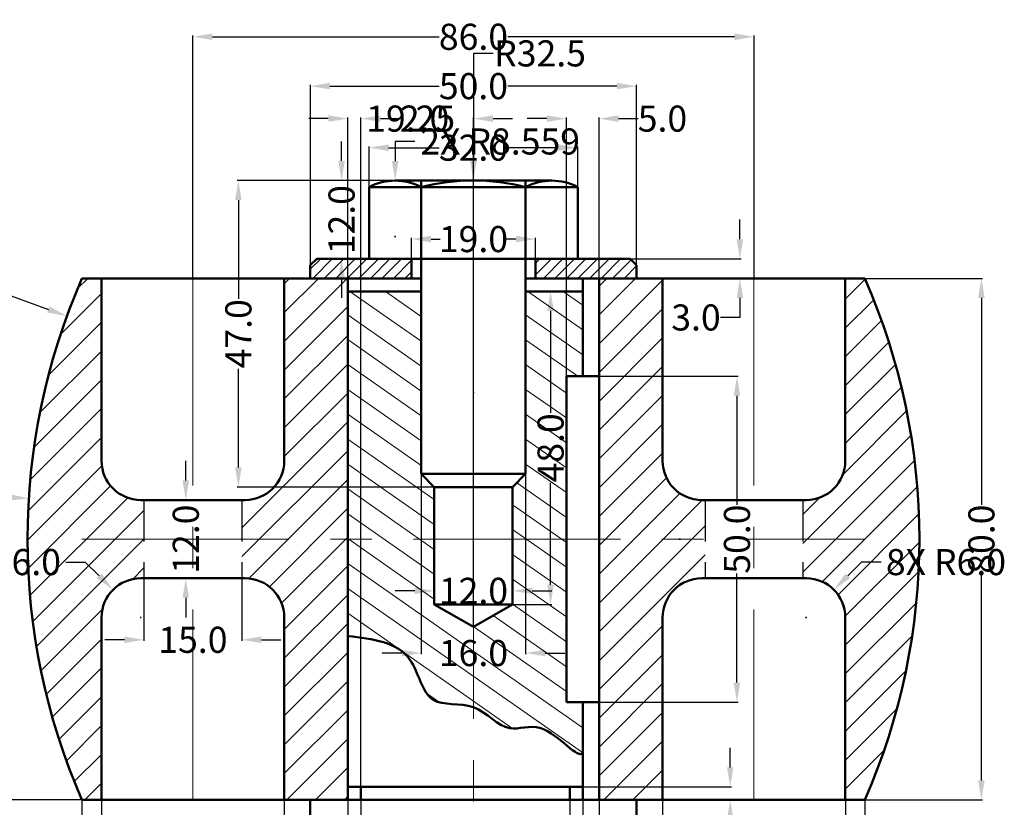
# Model space of a CAD drawing. Units: millimetres. Extents: x 285 to 514, y 588 to 771.
# Tile 3 of 3: x 363 to 514, y 650 to 771. Entities that reach past the tile are written whole.
import ezdxf

# ---------------------------------------------------------------- set-up
doc = ezdxf.new("R2010")
doc.units = ezdxf.units.MM
doc.header["$MEASUREMENT"] = 0
doc.linetypes.add('CENTER', pattern=[50.8, 31.75, -6.35, 6.35, -6.35])
doc.linetypes.add('HIDDEN', pattern=[9.525, 6.35, -3.175])
for name, color, linetype, lineweight in [('M-CNTR', 1, 'CENTER', 18), ('M-DIMS', 2, 'Continuous', 25), ('M-HATC', 8, 'Continuous', 18), ('M-HIDN', 3, 'HIDDEN', 25), ('M-OUTL', 7, 'Continuous', 50)]:
    doc.layers.add(name, color=color, linetype=linetype, lineweight=lineweight)
doc.styles.get("Standard").update_dxf_attribs({"font": 'arial.ttf'})
doc.dimstyles.get("Standard").update_dxf_attribs({"dimtxt": 4, "dimasz": 3, "dimexe": 0.18, "dimexo": 0.0625, "dimgap": 0.09, "dimtad": 0, "dimtoh": 1, "dimdec": 1, "dimzin": 0, "dimdsep": 46, "dimtxsty": 'Standard', "dimcen": 0.09, "dimadec": 0, "dimazin": 0, "dimtfac": 1, "dimtdec": 1, "dimtofl": 0, "dimtmove": 0, "dimatfit": 3, "dimfxl": 1, "dimtolj": 1, "dimtzin": 0, "dimarcsym": 0})

# ---------------------------------------------------------------- blocks, each defined once
blk = doc.blocks.new('*D1')
at = {"layer": 'Defpoints', "color": 0, "transparency": 16777216}
for p in [(413.04, 651.15), (451.54, 651.15), (451.54, 632.52)]:
    blk.add_point(p, dxfattribs=at)
at = {"layer": 'M-DIMS', "color": 0, "lineweight": -2, "transparency": 16777216}
for p, q in [((413.04, 651.09), (413.04, 632.34)), ((451.54, 651.09), (451.54, 632.34)), ((416.04, 632.52), (426.99, 632.52)), ((448.54, 632.52), (437.59, 632.52))]:
    blk.add_line(p, q, dxfattribs=at)
at = {"layer": 'M-DIMS', "color": 0, "transparency": 16777216}
for points in [[(416.04, 633.02), (416.04, 632.02), (413.04, 632.52)], [(448.54, 633.02), (448.54, 632.02), (451.54, 632.52)]]:
    blk.add_solid(points, dxfattribs=at)
at = {"layer": 'M-DIMS', "color": 0, "transparency": 16777216, "insert": (432.29, 632.52), "char_height": 4, "attachment_point": 5}
blk.add_mtext('\\A1;38.5', dxfattribs=at)
blk = doc.blocks.new('*D2')
at = {"layer": 'Defpoints', "color": 0, "transparency": 16777216}
for p in [(449.04, 656.31), (413.04, 648.81), (449.04, 638.14)]:
    blk.add_point(p, dxfattribs=at)
at = {"layer": 'M-DIMS', "color": 0, "lineweight": -2, "transparency": 16777216}
for p, q in [((449.04, 656.25), (449.04, 637.96)), ((413.04, 648.75), (413.04, 637.96)), ((416.04, 638.14), (425.76, 638.14)), ((446.04, 638.14), (436.31, 638.14))]:
    blk.add_line(p, q, dxfattribs=at)
at = {"layer": 'M-DIMS', "color": 0, "transparency": 16777216}
for points in [[(416.04, 638.64), (416.04, 637.64), (413.04, 638.14)], [(446.04, 638.64), (446.04, 637.64), (449.04, 638.14)]]:
    blk.add_solid(points, dxfattribs=at)
at = {"layer": 'M-DIMS', "color": 0, "transparency": 16777216, "insert": (431.04, 638.14), "char_height": 4, "attachment_point": 5}
blk.add_mtext('\\A1;36.0', dxfattribs=at)
blk = doc.blocks.new('*D3')
at = {"layer": 'Defpoints', "color": 0, "transparency": 16777216}
for p in [(364.13, 697.39), (463.94, 691.15)]:
    blk.add_point(p, dxfattribs=at)
at = {"layer": 'M-DIMS', "color": 0, "lineweight": -2, "transparency": 16777216}
for p, q in [((337.25, 699.07), (361.14, 697.58)), ((463.94, 691.06), (463.94, 691.24)), ((463.85, 691.15), (464.03, 691.15))]:
    blk.add_line(p, q, dxfattribs=at)
at = {"layer": 'M-DIMS', "color": 0, "transparency": 16777216}
blk.add_solid([(361.17, 698.07), (361.11, 697.08), (364.13, 697.39)], dxfattribs=at)
at = {"layer": 'M-DIMS', "color": 0, "transparency": 16777216, "insert": (328.5, 699.07), "char_height": 4, "attachment_point": 5}
blk.add_mtext('\\A1;R100.0', dxfattribs=at)
blk = doc.blocks.new('*D4')
at = {"layer": 'Defpoints', "color": 0, "transparency": 16777216}
for p in [(372.29, 651.15), (492.29, 651.15), (492.29, 590.54)]:
    blk.add_point(p, dxfattribs=at)
at = {"layer": 'M-DIMS', "color": 0, "lineweight": -2, "transparency": 16777216}
for p, q in [((372.29, 651.09), (372.29, 590.36)), ((492.29, 651.09), (492.29, 590.36)), ((375.29, 590.54), (425.64, 590.54)), ((489.29, 590.54), (438.93, 590.54))]:
    blk.add_line(p, q, dxfattribs=at)
at = {"layer": 'M-DIMS', "color": 0, "transparency": 16777216}
for points in [[(375.29, 591.04), (375.29, 590.04), (372.29, 590.54)], [(489.29, 591.04), (489.29, 590.04), (492.29, 590.54)]]:
    blk.add_solid(points, dxfattribs=at)
at = {"layer": 'M-DIMS', "color": 0, "transparency": 16777216, "insert": (432.29, 590.54), "char_height": 4, "attachment_point": 5}
blk.add_mtext('\\A1;120.0', dxfattribs=at)
blk = doc.blocks.new('*D5')
at = {"layer": 'Defpoints', "color": 0, "transparency": 16777216}
for p in [(375.29, 651.15), (489.29, 651.15), (489.29, 598.24)]:
    blk.add_point(p, dxfattribs=at)
at = {"layer": 'M-DIMS', "color": 0, "lineweight": -2, "transparency": 16777216}
for p, q in [((375.29, 651.09), (375.29, 598.06)), ((489.29, 651.09), (489.29, 598.06)), ((378.29, 598.24), (425.64, 598.24)), ((486.29, 598.24), (438.93, 598.24))]:
    blk.add_line(p, q, dxfattribs=at)
at = {"layer": 'M-DIMS', "color": 0, "transparency": 16777216}
for points in [[(378.29, 598.74), (378.29, 597.74), (375.29, 598.24)], [(486.29, 598.74), (486.29, 597.74), (489.29, 598.24)]]:
    blk.add_solid(points, dxfattribs=at)
at = {"layer": 'M-DIMS', "color": 0, "transparency": 16777216, "insert": (432.29, 598.24), "char_height": 4, "attachment_point": 5}
blk.add_mtext('\\A1;114.0', dxfattribs=at)
blk = doc.blocks.new('*D6')
at = {"layer": 'Defpoints', "color": 0, "transparency": 16777216}
for p in [(403.29, 651.15), (461.29, 651.15), (461.29, 604.76)]:
    blk.add_point(p, dxfattribs=at)
at = {"layer": 'M-DIMS', "color": 0, "lineweight": -2, "transparency": 16777216}
for p, q in [((403.29, 651.09), (403.29, 604.58)), ((461.29, 651.09), (461.29, 604.58)), ((406.29, 604.76), (427.01, 604.76)), ((458.29, 604.76), (437.57, 604.76))]:
    blk.add_line(p, q, dxfattribs=at)
at = {"layer": 'M-DIMS', "color": 0, "transparency": 16777216}
for points in [[(406.29, 605.26), (406.29, 604.26), (403.29, 604.76)], [(458.29, 605.26), (458.29, 604.26), (461.29, 604.76)]]:
    blk.add_solid(points, dxfattribs=at)
at = {"layer": 'M-DIMS', "color": 0, "transparency": 16777216, "insert": (432.29, 604.76), "char_height": 4, "attachment_point": 5}
blk.add_mtext('\\A1;58.0', dxfattribs=at)
blk = doc.blocks.new('*D8')
at = {"layer": 'Defpoints', "color": 0, "transparency": 16777216}
for p in [(415.04, 651.15), (447.04, 651.15), (447.04, 644.96)]:
    blk.add_point(p, dxfattribs=at)
at = {"layer": 'M-DIMS', "color": 0, "lineweight": -2, "transparency": 16777216}
for p, q in [((415.04, 651.09), (415.04, 644.78)), ((447.04, 651.09), (447.04, 644.78)), ((418.04, 644.96), (425.76, 644.96)), ((444.04, 644.96), (436.31, 644.96))]:
    blk.add_line(p, q, dxfattribs=at)
at = {"layer": 'M-DIMS', "color": 0, "transparency": 16777216}
for points in [[(418.04, 645.46), (418.04, 644.46), (415.04, 644.96)], [(444.04, 645.46), (444.04, 644.46), (447.04, 644.96)]]:
    blk.add_solid(points, dxfattribs=at)
at = {"layer": 'M-DIMS', "color": 0, "transparency": 16777216, "insert": (431.04, 644.96), "char_height": 4, "attachment_point": 5}
blk.add_mtext('\\A1;32.0', dxfattribs=at)
blk = doc.blocks.new('*D9')
at = {"layer": 'Defpoints', "color": 0, "transparency": 16777216}
for p in [(381.79, 685.15), (396.79, 685.15), (396.79, 675.71)]:
    blk.add_point(p, dxfattribs=at)
at = {"layer": 'M-DIMS', "color": 0, "lineweight": -2, "transparency": 16777216}
for p, q in [((381.79, 685.09), (381.79, 675.53)), ((396.79, 685.09), (396.79, 675.53)), ((378.79, 675.71), (375.79, 675.71)), ((399.79, 675.71), (402.79, 675.71))]:
    blk.add_line(p, q, dxfattribs=at)
at = {"layer": 'M-DIMS', "color": 0, "transparency": 16777216}
for points in [[(378.79, 676.21), (378.79, 675.21), (381.79, 675.71)], [(399.79, 676.21), (399.79, 675.21), (396.79, 675.71)]]:
    blk.add_solid(points, dxfattribs=at)
at = {"layer": 'M-DIMS', "color": 0, "transparency": 16777216, "insert": (389.29, 675.71), "char_height": 4, "attachment_point": 5}
blk.add_mtext('\\A1;15.0', dxfattribs=at)
blk = doc.blocks.new('*D10')
at = {"layer": 'Defpoints', "color": 0, "transparency": 16777216}
for p in [(424.29, 746.15), (412.07, 734.15), (424.29, 734.15)]:
    blk.add_point(p, dxfattribs=at)
at = {"layer": 'M-DIMS', "color": 0, "lineweight": -2, "transparency": 16777216}
for p, q in [((412.07, 749.15), (412.07, 752.15)), ((424.22, 746.15), (411.89, 746.15)), ((424.22, 734.15), (411.89, 734.15)), ((412.07, 731.15), (412.07, 728.15))]:
    blk.add_line(p, q, dxfattribs=at)
at = {"layer": 'M-DIMS', "color": 0, "transparency": 16777216}
for points in [[(411.57, 749.15), (412.57, 749.15), (412.07, 746.15)], [(411.57, 731.15), (412.57, 731.15), (412.07, 734.15)]]:
    blk.add_solid(points, dxfattribs=at)
at = {"layer": 'M-DIMS', "color": 0, "transparency": 16777216, "insert": (412.07, 740.15), "char_height": 4, "attachment_point": 5, "rotation": 90}
blk.add_mtext('\\A1;12.0', dxfattribs=at)
blk = doc.blocks.new('*D11')
at = {"layer": 'Defpoints', "color": 0, "transparency": 16777216}
for p in [(416.29, 746.15), (396.26, 699.14), (426.29, 699.14)]:
    blk.add_point(p, dxfattribs=at)
at = {"layer": 'M-DIMS', "color": 0, "lineweight": -2, "transparency": 16777216}
for p, q in [((416.23, 746.15), (396.08, 746.15)), ((396.26, 743.15), (396.26, 728)), ((396.26, 702.14), (396.26, 717.29)), ((426.22, 699.14), (396.08, 699.14))]:
    blk.add_line(p, q, dxfattribs=at)
at = {"layer": 'M-DIMS', "color": 0, "transparency": 16777216}
for points in [[(395.76, 743.15), (396.76, 743.15), (396.26, 746.15)], [(395.76, 702.14), (396.76, 702.14), (396.26, 699.14)]]:
    blk.add_solid(points, dxfattribs=at)
at = {"layer": 'M-DIMS', "color": 0, "transparency": 16777216, "insert": (396.26, 722.65), "char_height": 4, "attachment_point": 5, "rotation": 90}
blk.add_mtext('\\A1;47.0', dxfattribs=at)
blk = doc.blocks.new('*D12')
at = {"layer": 'Defpoints', "color": 0, "transparency": 16777216}
for p in [(475.29, 768.2), (389.29, 731.15), (475.29, 731.15)]:
    blk.add_point(p, dxfattribs=at)
at = {"layer": 'M-DIMS', "color": 0, "lineweight": -2, "transparency": 16777216}
for p, q in [((389.29, 731.21), (389.29, 768.38)), ((392.29, 768.2), (427.01, 768.2)), ((472.29, 768.2), (437.57, 768.2)), ((475.29, 731.21), (475.29, 768.38))]:
    blk.add_line(p, q, dxfattribs=at)
at = {"layer": 'M-DIMS', "color": 0, "transparency": 16777216}
for points in [[(392.29, 768.7), (392.29, 767.7), (389.29, 768.2)], [(472.29, 768.7), (472.29, 767.7), (475.29, 768.2)]]:
    blk.add_solid(points, dxfattribs=at)
at = {"layer": 'M-DIMS', "color": 0, "transparency": 16777216, "insert": (432.29, 768.2), "char_height": 4, "attachment_point": 5}
blk.add_mtext('\\A1;86.0', dxfattribs=at)
blk = doc.blocks.new('*D13')
at = {"layer": 'Defpoints', "color": 0, "transparency": 16777216}
for p in [(448.29, 751.19), (416.29, 742.48), (448.29, 742.48)]:
    blk.add_point(p, dxfattribs=at)
at = {"layer": 'M-DIMS', "color": 0, "lineweight": -2, "transparency": 16777216}
for p, q in [((416.29, 742.54), (416.29, 751.37)), ((419.29, 751.19), (427.01, 751.19)), ((445.29, 751.19), (437.56, 751.19)), ((448.29, 742.54), (448.29, 751.37))]:
    blk.add_line(p, q, dxfattribs=at)
at = {"layer": 'M-DIMS', "color": 0, "transparency": 16777216}
for points in [[(419.29, 751.69), (419.29, 750.69), (416.29, 751.19)], [(445.29, 751.69), (445.29, 750.69), (448.29, 751.19)]]:
    blk.add_solid(points, dxfattribs=at)
at = {"layer": 'M-DIMS', "color": 0, "transparency": 16777216, "insert": (432.29, 751.19), "char_height": 4, "attachment_point": 5}
blk.add_mtext('\\A1;32.0', dxfattribs=at)
blk = doc.blocks.new('*D14')
at = {"layer": 'Defpoints', "color": 0, "transparency": 16777216}
for p in [(457.29, 760.63), (407.29, 731.15), (457.29, 731.15)]:
    blk.add_point(p, dxfattribs=at)
at = {"layer": 'M-DIMS', "color": 0, "lineweight": -2, "transparency": 16777216}
for p, q in [((407.29, 731.21), (407.29, 760.81)), ((410.29, 760.63), (427.01, 760.63)), ((454.29, 760.63), (437.57, 760.63)), ((457.29, 731.21), (457.29, 760.81))]:
    blk.add_line(p, q, dxfattribs=at)
at = {"layer": 'M-DIMS', "color": 0, "transparency": 16777216}
for points in [[(410.29, 761.13), (410.29, 760.13), (407.29, 760.63)], [(454.29, 761.13), (454.29, 760.13), (457.29, 760.63)]]:
    blk.add_solid(points, dxfattribs=at)
at = {"layer": 'M-DIMS', "color": 0, "transparency": 16777216, "insert": (432.29, 760.63), "char_height": 4, "attachment_point": 5}
blk.add_mtext('\\A1;50.0', dxfattribs=at)
blk = doc.blocks.new('*D15')
at = {"layer": 'Defpoints', "color": 0, "transparency": 16777216}
for p in [(444.66, 729.15), (438.29, 681.15), (444.11, 681.15)]:
    blk.add_point(p, dxfattribs=at)
at = {"layer": 'M-DIMS', "color": 0, "lineweight": -2, "transparency": 16777216}
for p, q in [((444.6, 729.15), (443.93, 729.15)), ((444.11, 726.15), (444.11, 710.51)), ((444.11, 684.15), (444.11, 699.79)), ((438.35, 681.15), (444.29, 681.15))]:
    blk.add_line(p, q, dxfattribs=at)
at = {"layer": 'M-DIMS', "color": 0, "transparency": 16777216}
for points in [[(443.61, 726.15), (444.61, 726.15), (444.11, 729.15)], [(443.61, 684.15), (444.61, 684.15), (444.11, 681.15)]]:
    blk.add_solid(points, dxfattribs=at)
at = {"layer": 'M-DIMS', "color": 0, "transparency": 16777216, "insert": (444.11, 705.15), "char_height": 4, "attachment_point": 5, "rotation": 90}
blk.add_mtext('\\A1;48.0', dxfattribs=at)
blk = doc.blocks.new('*D16')
at = {"layer": 'Defpoints', "color": 0, "transparency": 16777216}
for p in [(424.29, 701.14), (440.29, 701.14), (440.29, 673.68)]:
    blk.add_point(p, dxfattribs=at)
at = {"layer": 'M-DIMS', "color": 0, "lineweight": -2, "transparency": 16777216}
for p, q in [((424.29, 701.08), (424.29, 673.5)), ((440.29, 701.08), (440.29, 673.5)), ((421.29, 673.68), (418.29, 673.68)), ((443.29, 673.68), (446.29, 673.68))]:
    blk.add_line(p, q, dxfattribs=at)
at = {"layer": 'M-DIMS', "color": 0, "transparency": 16777216}
for points in [[(421.29, 674.18), (421.29, 673.18), (424.29, 673.68)], [(443.29, 674.18), (443.29, 673.18), (440.29, 673.68)]]:
    blk.add_solid(points, dxfattribs=at)
at = {"layer": 'M-DIMS', "color": 0, "transparency": 16777216, "insert": (432.29, 673.68), "char_height": 4, "attachment_point": 5}
blk.add_mtext('\\A1;16.0', dxfattribs=at)
blk = doc.blocks.new('*D17')
at = {"layer": 'Defpoints', "color": 0, "transparency": 16777216}
for p in [(438.29, 683.22), (426.29, 681.15), (438.29, 681.15)]:
    blk.add_point(p, dxfattribs=at)
at = {"layer": 'M-DIMS', "color": 0, "lineweight": -2, "transparency": 16777216}
for p, q in [((423.29, 683.22), (420.29, 683.22)), ((426.29, 681.21), (426.29, 683.4)), ((438.29, 681.21), (438.29, 683.4)), ((441.29, 683.22), (444.29, 683.22))]:
    blk.add_line(p, q, dxfattribs=at)
at = {"layer": 'M-DIMS', "color": 0, "transparency": 16777216}
for points in [[(423.29, 683.72), (423.29, 682.72), (426.29, 683.22)], [(441.29, 683.72), (441.29, 682.72), (438.29, 683.22)]]:
    blk.add_solid(points, dxfattribs=at)
at = {"layer": 'M-DIMS', "color": 0, "transparency": 16777216, "insert": (432.29, 683.22), "char_height": 4, "attachment_point": 5}
blk.add_mtext('\\A1;12.0', dxfattribs=at)
blk = doc.blocks.new('*D18')
at = {"layer": 'Defpoints', "color": 0, "transparency": 16777216}
for p in [(451.54, 716.15), (451.54, 666.15), (472.68, 666.15)]:
    blk.add_point(p, dxfattribs=at)
at = {"layer": 'M-DIMS', "color": 0, "lineweight": -2, "transparency": 16777216}
for p, q in [((451.6, 716.15), (472.86, 716.15)), ((472.68, 713.15), (472.68, 696.43)), ((472.68, 669.15), (472.68, 685.87)), ((451.6, 666.15), (472.86, 666.15))]:
    blk.add_line(p, q, dxfattribs=at)
at = {"layer": 'M-DIMS', "color": 0, "transparency": 16777216}
for points in [[(472.18, 713.15), (473.18, 713.15), (472.68, 716.15)], [(472.18, 669.15), (473.18, 669.15), (472.68, 666.15)]]:
    blk.add_solid(points, dxfattribs=at)
at = {"layer": 'M-DIMS', "color": 0, "transparency": 16777216, "insert": (472.68, 691.15), "char_height": 4, "attachment_point": 5, "rotation": 90}
blk.add_mtext('\\A1;50.0', dxfattribs=at)
blk = doc.blocks.new('*D19')
at = {"layer": 'Defpoints', "color": 0, "transparency": 16777216}
for p in [(449.04, 653.15), (449.04, 651.15), (471.64, 651.15)]:
    blk.add_point(p, dxfattribs=at)
at = {"layer": 'M-DIMS', "color": 0, "lineweight": -2, "transparency": 16777216}
for p, q in [((471.64, 656.15), (471.64, 659.15)), ((449.1, 653.15), (471.82, 653.15)), ((449.1, 651.15), (471.82, 651.15)), ((471.64, 648.15), (471.64, 645.15)), ((471.64, 645.15), (468.64, 645.15))]:
    blk.add_line(p, q, dxfattribs=at)
at = {"layer": 'M-DIMS', "color": 0, "transparency": 16777216}
for points in [[(471.14, 656.15), (472.14, 656.15), (471.64, 653.15)], [(471.14, 648.15), (472.14, 648.15), (471.64, 651.15)]]:
    blk.add_solid(points, dxfattribs=at)
at = {"layer": 'M-DIMS', "color": 0, "transparency": 16777216, "insert": (464.88, 645.15), "char_height": 4, "attachment_point": 5}
blk.add_mtext('\\A1;2.0', dxfattribs=at)
blk = doc.blocks.new('*D20')
at = {"layer": 'Defpoints', "color": 0, "transparency": 16777216}
for p in [(455.38, 734.15), (455.38, 731.15), (473.13, 731.15)]:
    blk.add_point(p, dxfattribs=at)
at = {"layer": 'M-DIMS', "color": 0, "lineweight": -2, "transparency": 16777216}
for p, q in [((473.13, 737.15), (473.13, 740.15)), ((455.44, 734.15), (473.31, 734.15)), ((455.44, 731.15), (473.31, 731.15)), ((473.13, 728.15), (473.13, 725.15)), ((473.13, 725.15), (470.13, 725.15))]:
    blk.add_line(p, q, dxfattribs=at)
at = {"layer": 'M-DIMS', "color": 0, "transparency": 16777216}
for points in [[(472.63, 737.15), (473.63, 737.15), (473.13, 734.15)], [(472.63, 728.15), (473.63, 728.15), (473.13, 731.15)]]:
    blk.add_solid(points, dxfattribs=at)
at = {"layer": 'M-DIMS', "color": 0, "transparency": 16777216, "insert": (466.4, 725.15), "char_height": 4, "attachment_point": 5}
blk.add_mtext('\\A1;3.0', dxfattribs=at)
blk = doc.blocks.new('*D21')
at = {"layer": 'Defpoints', "color": 0, "transparency": 16777216}
for p in [(441.79, 737.17), (422.79, 732.58), (441.79, 732.65)]:
    blk.add_point(p, dxfattribs=at)
at = {"layer": 'M-DIMS', "color": 0, "lineweight": -2, "transparency": 16777216}
for p, q in [((422.79, 732.64), (422.79, 737.35)), ((425.79, 737.17), (427.2, 737.17)), ((438.79, 737.17), (437.38, 737.17)), ((441.79, 732.71), (441.79, 737.35))]:
    blk.add_line(p, q, dxfattribs=at)
at = {"layer": 'M-DIMS', "color": 0, "transparency": 16777216}
for points in [[(425.79, 737.67), (425.79, 736.67), (422.79, 737.17)], [(438.79, 737.67), (438.79, 736.67), (441.79, 737.17)]]:
    blk.add_solid(points, dxfattribs=at)
at = {"layer": 'M-DIMS', "color": 0, "transparency": 16777216, "insert": (432.29, 737.17), "char_height": 4, "attachment_point": 5}
blk.add_mtext('\\A1;19.0', dxfattribs=at)
blk = doc.blocks.new('*D22')
at = {"layer": 'Defpoints', "color": 0, "transparency": 16777216}
for p in [(387.79, 697.15), (387.79, 685.15), (388.2, 685.15)]:
    blk.add_point(p, dxfattribs=at)
at = {"layer": 'M-DIMS', "color": 0, "lineweight": -2, "transparency": 16777216}
for p, q in [((388.2, 700.15), (388.2, 703.15)), ((387.85, 697.15), (388.38, 697.15)), ((387.85, 685.15), (388.38, 685.15)), ((388.2, 682.15), (388.2, 679.15))]:
    blk.add_line(p, q, dxfattribs=at)
at = {"layer": 'M-DIMS', "color": 0, "transparency": 16777216}
for points in [[(387.7, 700.15), (388.7, 700.15), (388.2, 697.15)], [(387.7, 682.15), (388.7, 682.15), (388.2, 685.15)]]:
    blk.add_solid(points, dxfattribs=at)
at = {"layer": 'M-DIMS', "color": 0, "transparency": 16777216, "insert": (388.2, 691.15), "char_height": 4, "attachment_point": 5, "rotation": 90}
blk.add_mtext('\\A1;12.0', dxfattribs=at)
blk = doc.blocks.new('*D23')
at = {"layer": 'Defpoints', "color": 0, "transparency": 16777216}
for p in [(407.29, 651.15), (354.44, 626.15), (407.29, 626.15)]:
    blk.add_point(p, dxfattribs=at)
at = {"layer": 'M-DIMS', "color": 0, "lineweight": -2, "transparency": 16777216}
for p, q in [((407.22, 651.15), (354.26, 651.15)), ((354.44, 648.15), (354.44, 643.96)), ((354.44, 629.15), (354.44, 633.34)), ((407.22, 626.15), (354.26, 626.15))]:
    blk.add_line(p, q, dxfattribs=at)
at = {"layer": 'M-DIMS', "color": 0, "transparency": 16777216}
for points in [[(353.94, 648.15), (354.94, 648.15), (354.44, 651.15)], [(353.94, 629.15), (354.94, 629.15), (354.44, 626.15)]]:
    blk.add_solid(points, dxfattribs=at)
at = {"layer": 'M-DIMS', "color": 0, "transparency": 16777216, "insert": (354.44, 638.65), "char_height": 4, "attachment_point": 5, "rotation": 90}
blk.add_mtext('\\A1;25.0', dxfattribs=at)
blk = doc.blocks.new('*D24')
at = {"layer": 'Defpoints', "color": 0, "transparency": 16777216}
for p in [(451.54, 755.65), (446.54, 716.15), (451.54, 716.15)]:
    blk.add_point(p, dxfattribs=at)
at = {"layer": 'M-DIMS', "color": 0, "lineweight": -2, "transparency": 16777216}
for p, q in [((443.54, 755.65), (440.54, 755.65)), ((446.54, 716.21), (446.54, 755.83)), ((451.54, 716.21), (451.54, 755.83)), ((454.54, 755.65), (457.54, 755.65))]:
    blk.add_line(p, q, dxfattribs=at)
at = {"layer": 'M-DIMS', "color": 0, "transparency": 16777216}
for points in [[(443.54, 756.15), (443.54, 755.15), (446.54, 755.65)], [(454.54, 756.15), (454.54, 755.15), (451.54, 755.65)]]:
    blk.add_solid(points, dxfattribs=at)
at = {"layer": 'M-DIMS', "color": 0, "transparency": 16777216, "insert": (461.26, 755.65), "char_height": 4, "attachment_point": 5}
blk.add_mtext('\\A1;5.0', dxfattribs=at)
blk = doc.blocks.new('*D25')
at = {"layer": 'Defpoints', "color": 0, "transparency": 16777216}
for p in [(492.29, 731.15), (492.29, 651.15), (510.14, 651.15)]:
    blk.add_point(p, dxfattribs=at)
at = {"layer": 'M-DIMS', "color": 0, "lineweight": -2, "transparency": 16777216}
for p, q in [((492.35, 731.15), (510.32, 731.15)), ((510.14, 728.15), (510.14, 696.43)), ((510.14, 654.15), (510.14, 685.87)), ((492.35, 651.15), (510.32, 651.15))]:
    blk.add_line(p, q, dxfattribs=at)
at = {"layer": 'M-DIMS', "color": 0, "transparency": 16777216}
for points in [[(509.64, 728.15), (510.64, 728.15), (510.14, 731.15)], [(509.64, 654.15), (510.64, 654.15), (510.14, 651.15)]]:
    blk.add_solid(points, dxfattribs=at)
at = {"layer": 'M-DIMS', "color": 0, "transparency": 16777216, "insert": (510.14, 691.15), "char_height": 4, "attachment_point": 5, "rotation": 90}
blk.add_mtext('\\A1;80.0', dxfattribs=at)
blk = doc.blocks.new('*D26')
at = {"layer": 'Defpoints', "color": 0, "transparency": 16777216}
for p in [(432.29, 746.15), (432.29, 713.65)]:
    blk.add_point(p, dxfattribs=at)
at = {"layer": 'M-DIMS', "color": 0, "lineweight": -2, "transparency": 16777216}
for p, q in [((435.29, 765.65), (432.29, 765.65)), ((432.29, 765.65), (432.29, 749.15)), ((432.2, 713.65), (432.38, 713.65)), ((432.29, 713.56), (432.29, 713.74))]:
    blk.add_line(p, q, dxfattribs=at)
at = {"layer": 'M-DIMS', "color": 0, "transparency": 16777216}
blk.add_solid([(431.79, 749.15), (432.79, 749.15), (432.29, 746.15)], dxfattribs=at)
at = {"layer": 'M-DIMS', "color": 0, "transparency": 16777216, "insert": (442.5, 765.65), "char_height": 4, "attachment_point": 5}
blk.add_mtext('\\A1;R32.5', dxfattribs=at)
blk = doc.blocks.new('*D27')
at = {"layer": 'Defpoints', "color": 0, "transparency": 16777216}
for p in [(420.29, 746.14), (420.29, 737.58)]:
    blk.add_point(p, dxfattribs=at)
at = {"layer": 'M-DIMS', "color": 0, "lineweight": -2, "transparency": 16777216}
for p, q in [((423.29, 752.14), (420.29, 752.14)), ((420.29, 752.14), (420.29, 749.14)), ((420.2, 737.58), (420.38, 737.58)), ((420.29, 737.49), (420.29, 737.67))]:
    blk.add_line(p, q, dxfattribs=at)
at = {"layer": 'M-DIMS', "color": 0, "transparency": 16777216}
blk.add_solid([(419.79, 749.14), (420.79, 749.14), (420.29, 746.14)], dxfattribs=at)
at = {"layer": 'M-DIMS', "color": 0, "transparency": 16777216, "insert": (436.38, 752.14), "char_height": 4, "attachment_point": 5}
blk.add_mtext('\\A1;2X R8.559', dxfattribs=at)
blk = doc.blocks.new('*D30')
at = {"layer": 'Defpoints', "color": 0, "transparency": 16777216}
for p in [(377.04, 683.39), (381.29, 679.15)]:
    blk.add_point(p, dxfattribs=at)
at = {"layer": 'M-DIMS', "color": 0, "lineweight": -2, "transparency": 16777216}
for p, q in [((369.8, 687.63), (372.8, 687.63)), ((372.8, 687.63), (374.92, 685.51)), ((381.2, 679.15), (381.38, 679.15)), ((381.29, 679.06), (381.29, 679.24))]:
    blk.add_line(p, q, dxfattribs=at)
at = {"layer": 'M-DIMS', "color": 0, "transparency": 16777216}
blk.add_solid([(375.28, 685.87), (374.57, 685.16), (377.04, 683.39)], dxfattribs=at)
at = {"layer": 'M-DIMS', "color": 0, "transparency": 16777216, "insert": (359.86, 687.63), "char_height": 4, "attachment_point": 5}
blk.add_mtext('\\A1;8X R6.0', dxfattribs=at)
blk = doc.blocks.new('*D31')
at = {"layer": 'Defpoints', "color": 0, "transparency": 16777216}
for p in [(432.286926, 755.649229), (432.286926, 677.685127), (413.036926, 653.149229)]:
    blk.add_point(p, dxfattribs=at)
at = {"layer": 'M-DIMS', "color": 0, "lineweight": -2, "transparency": 16777216}
for p, q in [((410.036926, 755.649229), (407.036926, 755.649229)), ((413.036926, 653.211729), (413.036926, 755.829229)), ((432.286926, 677.747627), (432.286926, 755.829229)), ((435.286926, 755.649229), (438.286926, 755.649229))]:
    blk.add_line(p, q, dxfattribs=at)
at = {"layer": 'M-DIMS', "color": 0, "transparency": 16777216}
for points in [[(410.036926, 756.149229), (410.036926, 755.149229), (413.036926, 755.649229)], [(435.286926, 756.149229), (435.286926, 755.149229), (432.286926, 755.649229)]]:
    blk.add_solid(points, dxfattribs=at)
at = {"layer": 'M-DIMS', "color": 0, "transparency": 16777216, "insert": (422.661926, 755.649229), "char_height": 4, "attachment_point": 5}
blk.add_mtext('\\A1;19.25', dxfattribs=at)
blk = doc.blocks.new('*D32')
at = {"layer": 'Defpoints', "color": 0, "transparency": 16777216}
for p in [(415.04, 755.65), (413.04, 653.15), (415.04, 653.15)]:
    blk.add_point(p, dxfattribs=at)
at = {"layer": 'M-DIMS', "color": 0, "lineweight": -2, "transparency": 16777216}
for p, q in [((410.04, 755.65), (407.04, 755.65)), ((413.04, 653.21), (413.04, 755.83)), ((415.04, 653.21), (415.04, 755.83)), ((418.04, 755.65), (421.04, 755.65))]:
    blk.add_line(p, q, dxfattribs=at)
at = {"layer": 'M-DIMS', "color": 0, "transparency": 16777216}
for points in [[(410.04, 756.15), (410.04, 755.15), (413.04, 755.65)], [(418.04, 756.15), (418.04, 755.15), (415.04, 755.65)]]:
    blk.add_solid(points, dxfattribs=at)
at = {"layer": 'M-DIMS', "color": 0, "transparency": 16777216, "insert": (424.8, 755.65), "char_height": 4, "attachment_point": 5}
blk.add_mtext('\\A1;2.0', dxfattribs=at)
blk = doc.blocks.new('*D33')
at = {"layer": 'Defpoints', "color": 0, "transparency": 16777216}
for p in [(369.97, 725.35), (463.94, 691.15)]:
    blk.add_point(p, dxfattribs=at)
at = {"layer": 'M-DIMS', "color": 0, "lineweight": -2, "transparency": 16777216}
for p, q in [((310.59, 745.87), (313.59, 745.87)), ((313.59, 745.87), (367.15, 726.38)), ((463.94, 691.06), (463.94, 691.24)), ((463.85, 691.15), (464.03, 691.15))]:
    blk.add_line(p, q, dxfattribs=at)
at = {"layer": 'M-DIMS', "color": 0, "transparency": 16777216}
blk.add_solid([(367.32, 726.85), (366.98, 725.91), (369.97, 725.35)], dxfattribs=at)
at = {"layer": 'M-DIMS', "color": 0, "transparency": 16777216, "insert": (297.51, 745.87), "char_height": 4, "attachment_point": 5}
blk.add_mtext('\\A1;2X R100.0', dxfattribs=at)
blk = doc.blocks.new('*D35')
at = {"layer": 'Defpoints', "color": 0, "transparency": 16777216}
for p in [(487.53, 683.39), (483.29, 679.15)]:
    blk.add_point(p, dxfattribs=at)
at = {"layer": 'M-DIMS', "color": 0, "lineweight": -2, "transparency": 16777216}
for p, q in [((491.77, 687.63), (489.65, 685.51)), ((494.77, 687.63), (491.77, 687.63)), ((483.2, 679.15), (483.38, 679.15)), ((483.29, 679.06), (483.29, 679.24))]:
    blk.add_line(p, q, dxfattribs=at)
at = {"layer": 'M-DIMS', "color": 0, "transparency": 16777216}
blk.add_solid([(489.3, 685.87), (490.01, 685.16), (487.53, 683.39)], dxfattribs=at)
at = {"layer": 'M-DIMS', "color": 0, "transparency": 16777216, "insert": (504.71, 687.63), "char_height": 4, "attachment_point": 5}
blk.add_mtext('\\A1;8X R6.0', dxfattribs=at)

msp = doc.modelspace()

# ---------------------------------------------------------------- hatches: boundary and pattern name
at = {"layer": 'M-HATC'}
h = msp.add_hatch(dxfattribs=at)
h.set_pattern_fill('ANSI31', color=256, scale=10)
h.paths.add_polyline_path([(422.7869, 734.1492), (408.2869, 734.1492), (407.2869, 733.1492), (407.2869, 731.1492), (422.7869, 731.1492)])
h.paths.add_polyline_path([(457.2869, 733.1492), (456.2869, 734.1492), (441.7869, 734.1492), (441.7869, 731.1492), (457.2869, 731.1492)])
h = msp.add_hatch(dxfattribs=at)
h.set_pattern_fill('ANSI31', color=256, scale=25)
h.paths.add_polyline_path([(381.7869, 697.1492), (381.2869, 697.1492, -0.41421356), (375.2869, 703.1492), (375.2869, 731.1492), (372.2869, 731.1492, 0.20871215), (372.2869, 651.1492), (375.2869, 651.1492), (375.2869, 679.1492, -0.41421356), (381.2869, 685.1492), (381.7869, 685.1492)])
h.paths.add_polyline_path([(413.0369, 691.1492), (396.7869, 691.1492), (396.7869, 685.1492), (397.2869, 685.1492, -0.41421356), (403.2869, 679.1492), (403.2869, 651.1492), (413.0369, 651.1492)])
h.paths.add_polyline_path([(413.0369, 731.1492), (403.2869, 731.1492), (403.2869, 703.1492, -0.41421356), (397.2869, 697.1492), (396.7869, 697.1492), (396.7869, 691.1492), (413.0369, 691.1492)])
h.paths.add_polyline_path([(467.7869, 697.1492), (467.2869, 697.1492, -0.41421356), (461.2869, 703.1492), (461.2869, 731.1492), (451.5369, 731.1492), (451.5369, 691.1492), (467.7869, 691.1492)])
h.paths.add_polyline_path([(467.2869, 685.1492), (467.7869, 685.1492), (467.7869, 691.1492), (451.5369, 691.1492), (451.5369, 651.1492), (461.2869, 651.1492), (461.2869, 679.1492, -0.41421356)])
h.paths.add_polyline_path([(492.2869, 731.1492), (489.2869, 731.1492), (489.2869, 703.1492, -0.41421356), (483.2869, 697.1492), (482.7869, 697.1492), (482.7869, 685.1492), (483.2869, 685.1492, -0.41421356), (489.2869, 679.1492), (489.2869, 651.1492), (492.2869, 651.1492, 0.20871215)])
h = msp.add_hatch(dxfattribs=at)
h.set_pattern_fill('ANSI31', color=256, scale=25, angle=100)
h.paths.add_polyline_path([(424.2869, 729.1492), (413.0369, 729.1492), (413.0369, 691.1492), (426.2869, 691.1492), (426.2869, 699.1414), (424.2869, 701.1414)])
edge = h.paths.add_edge_path()
edge.add_line((426.2869, 691.1492), (413.0369, 691.1492))
edge.add_line((413.0369, 691.1492), (413.0369, 676.2796))
edge.add_spline(control_points=[(413.0369, 676.2796), (416.8322, 675.8566), (423.2548, 675.1409), (424.7571, 664.892), (430.226, 666.109), (432.2869, 665.3573)], knot_values=[0, 0, 0, 0, 10.1994056, 17.25965485, 23.56109176, 23.56109176, 23.56109176, 23.56109176], degree=3, periodic=0)
edge.add_line((432.2869, 665.3573), (432.2869, 677.6851))
edge.add_line((432.2869, 677.6851), (426.2869, 681.1492))
edge.add_line((426.2869, 681.1492), (426.2869, 691.1492))
h.paths.add_polyline_path([(446.5369, 716.1492), (449.0369, 716.1492), (449.0369, 729.1492), (440.2869, 729.1492), (440.2869, 701.1414), (438.2869, 699.1414), (438.2869, 691.1492), (446.5369, 691.1492)])
h.paths.add_polyline_path([(432.2869, 665.3573), (432.6694, 665.2007), (433.0408, 665.0172), (433.4024, 664.8114), (433.7554, 664.5878), (434.1011, 664.3509), (434.4407, 664.1051), (434.7753, 663.8552), (435.1063, 663.6054), (435.4349, 663.3605), (435.7623, 663.1249), (436.0897, 662.903), (436.4183, 662.6995), (436.7494, 662.5189), (437.0843, 662.3657), (437.4241, 662.2443), (437.77, 662.1594), (438.1233, 662.1145), (438.4842, 662.1052), (438.8527, 662.1234), (439.2286, 662.161), (439.612, 662.2098), (440.0028, 662.2617), (440.4009, 662.3085), (440.8062, 662.3421), (441.2187, 662.3543), (441.6383, 662.337), (442.0649, 662.2819), (442.4985, 662.181), (442.9389, 662.0273), (443.3841, 661.8233), (443.8315, 661.5771), (444.2782, 661.2967), (444.7215, 660.9901), (445.1588, 660.6653), (445.5872, 660.3304), (446.0039, 659.9933), (446.4064, 659.6621), (446.7917, 659.3448), (447.1572, 659.0495), (447.5001, 658.784), (447.8176, 658.5565), (448.1071, 658.375), (448.3657, 658.2475), (448.5907, 658.182), (448.7795, 658.1865), (448.9291, 658.269), (449.0369, 658.4376), (449.0369, 666.1492), (446.5369, 666.1492), (446.5369, 691.1492), (438.2869, 691.1492), (438.2869, 681.1492), (432.2869, 677.6851)])

# ---------------------------------------------------------------- linework, layer by layer
at = {"layer": 'M-CNTR'}
for p, q in [((432.2869, 746.1492), (432.2869, 626.1492)), ((389.2869, 731.1492), (389.2869, 651.1492)), ((475.2869, 731.1492), (475.2869, 651.1492)), ((372.2869, 691.1492), (492.2869, 691.1492))]:
    msp.add_line(p, q, dxfattribs=at)
at = {"layer": 'M-HIDN'}
for p, q in [((381.7869, 697.1492), (381.7869, 685.1492)), ((396.7869, 697.1492), (396.7869, 685.1492)), ((467.7869, 697.1492), (467.7869, 685.1492)), ((482.7869, 697.1492), (482.7869, 685.1492))]:
    msp.add_line(p, q, dxfattribs=at)
at = {"layer": 'M-OUTL'}
for p, q in [((420.2869, 746.1414), (444.2869, 746.1414)), ((424.2869, 746.1492), (424.2869, 746.1414)), ((424.2869, 746.1492), (424.2869, 729.1492)), ((440.2869, 746.1492), (440.2869, 746.1414)), ((440.2869, 746.1492), (440.2869, 729.1492)), ((416.2869, 745.1492), (416.2869, 734.1492)), ((416.2869, 745.1492), (448.2869, 745.1492)), ((448.2869, 745.1492), (448.2869, 734.1492)), ((408.2869, 734.1492), (407.2869, 733.1492)), ((408.2869, 734.1492), (456.2869, 734.1492)), ((422.7869, 734.1492), (422.7869, 731.1492)), ((441.7869, 734.1492), (441.7869, 731.1492)), ((456.2869, 734.1492), (457.2869, 733.1492)), ((407.2869, 733.1492), (407.2869, 731.1492)), ((457.2869, 733.1492), (457.2869, 731.1492)), ((372.2869, 731.1492), (424.2869, 731.1492)), ((375.2869, 731.1492), (375.2869, 703.1492)), ((403.2869, 731.1492), (403.2869, 703.1492)), ((413.0369, 731.1492), (413.0369, 651.1492)), ((440.2869, 731.1492), (492.2869, 731.1492)), ((449.0369, 731.1492), (449.0369, 716.1492)), ((451.5369, 731.1492), (451.5369, 651.1492)), ((461.2869, 731.1492), (461.2869, 703.1492)), ((489.2869, 731.1492), (489.2869, 703.1492)), ((413.0369, 729.1492), (424.2869, 729.1492)), ((424.2869, 729.1492), (424.2869, 701.1414)), ((440.2869, 729.1492), (440.2869, 701.1414)), ((440.2869, 729.1492), (449.0369, 729.1492)), ((446.5369, 716.1492), (446.5369, 666.1492)), ((446.5369, 716.1492), (451.5369, 716.1492)), ((424.2869, 701.1414), (440.2869, 701.1414)), ((426.2869, 699.1414), (424.2869, 701.1414)), ((438.2869, 699.1414), (440.2869, 701.1414)), ((426.2869, 699.1414), (438.2869, 699.1414)), ((426.2869, 699.1414), (426.2869, 681.1492)), ((438.2869, 699.1414), (438.2869, 681.1492)), ((381.2869, 697.1492), (397.2869, 697.1492)), ((467.2869, 697.1492), (483.2869, 697.1492)), ((381.2869, 685.1492), (397.2869, 685.1492)), ((467.2869, 685.1492), (483.2869, 685.1492)), ((426.2869, 681.1492), (438.2869, 681.1492)), ((426.2869, 681.1492), (432.2869, 677.6851)), ((438.2869, 681.1492), (432.2869, 677.6851)), ((375.2869, 679.1492), (375.2869, 651.1492)), ((403.2869, 679.1492), (403.2869, 651.1492)), ((461.2869, 679.1492), (461.2869, 651.1492)), ((489.2869, 679.1492), (489.2869, 651.1492)), ((451.5369, 666.1492), (446.5369, 666.1492)), ((449.0369, 666.1492), (449.0369, 651.1492)), ((449.0369, 653.1492), (413.0369, 653.1492)), ((415.0369, 653.1492), (415.0369, 651.1492)), ((447.0369, 653.1492), (447.0369, 651.1492)), ((492.2869, 651.1492), (372.2869, 651.1492)), ((407.2869, 651.1492), (407.2869, 626.1492)), ((457.2869, 651.1492), (457.2869, 626.1492))]:
    msp.add_line(p, q, dxfattribs=at)
for centre, radius, start, end in [((420.2869, 737.5824), 8.559, 62.13791, 117.86209), ((432.2869, 713.6492), 32.5, 75.749967, 104.250033), ((444.2869, 737.5824), 8.559, 62.13791, 117.86209), ((463.9384, 691.1492), 100, 156.421822, 203.578178), ((400.6354, 691.1492), 100, 336.421822, 23.578178), ((381.2869, 703.1492), 6, 180, 270), ((397.2869, 703.1492), 6, 270, 0), ((467.2869, 703.1492), 6, 180, 270), ((483.2869, 703.1492), 6, 270, 0), ((381.2869, 679.1492), 6, 90, 180), ((397.2869, 679.1492), 6, 0, 90), ((467.2869, 679.1492), 6, 90, 180), ((483.2869, 679.1492), 6, 0, 90)]:
    msp.add_arc(centre, radius, start, end, dxfattribs=at)
msp.add_open_spline([(413.0369, 676.2796), (416.8322, 675.8566), (423.2548, 675.1409), (424.7571, 664.892), (432.855, 666.6941), (437.109, 660.8572), (443.3352, 663.941), (448.4998, 657.0993), (449.0369, 658.4376)], degree=3, knots=[0, 0, 0, 0, 10.1994056, 17.25965485, 23.56109176, 29.98433035, 34.74904808, 42.16522138, 42.16522138, 42.16522138, 42.16522138], dxfattribs=at)

# ---------------------------------------------------------------- dimensions: what is measured, and where the dimension line sits
at = {"layer": 'M-DIMS'}
for base, p1, p2, override, picture, middle in [((475.2869, 768.1977), (389.2869, 731.1492), (475.2869, 731.1492), {"dimclrd": 0, "dimclre": 0, "dimclrt": 0}, '*D12', (432.2869, 768.1977)), ((457.2869, 760.6331), (407.2869, 731.1492), (457.2869, 731.1492), {"dimclrd": 0, "dimclre": 0, "dimclrt": 0}, '*D14', (432.2869, 760.6331)), ((432.2869, 755.6492), (413.0369, 653.1492), (432.2869, 677.6851), {"dimdec": 2, "dimlfac": 1, "dimrnd": 0, "dimzin": 0, "dimdsep": 46, "dimlunit": 2}, '*D31', (422.6619, 755.6492)), ((415.0369, 755.6492), (413.0369, 653.1492), (415.0369, 653.1492), {"dimdec": 1, "dimlfac": 1, "dimrnd": 0, "dimzin": 0, "dimdsep": 46, "dimlunit": 2}, '*D32', (424.7954, 755.6492)), ((451.5369, 755.6492), (446.5369, 716.1492), (451.5369, 716.1492), {"dimdec": 1, "dimlfac": 1, "dimrnd": 0, "dimzin": 0, "dimdsep": 46, "dimlunit": 2}, '*D24', (461.2613, 755.6492)), ((448.2869, 751.1859), (416.2869, 742.4751), (448.2869, 742.4751), {"dimclrd": 0, "dimclre": 0, "dimclrt": 0}, '*D13', (432.2869, 751.1859)), ((441.7869, 737.1715), (422.7869, 732.5818), (441.7869, 732.6492), {"dimclrd": 0, "dimclre": 0, "dimclrt": 0}, '*D21', (432.2869, 737.1715)), ((440.2869, 673.6786), (424.2869, 701.1414), (440.2869, 701.1414), {"dimclrd": 0, "dimclre": 0, "dimclrt": 0}, '*D16', (432.2869, 673.6786)), ((396.7869, 675.713), (381.7869, 685.1492), (396.7869, 685.1492), {"dimclrd": 0, "dimclre": 0, "dimclrt": 0}, '*D9', (389.2869, 675.713)), ((438.2869, 683.2214), (426.2869, 681.1492), (438.2869, 681.1492), {"dimclrd": 0, "dimclre": 0, "dimclrt": 0}, '*D17', (432.2869, 683.2214)), ((449.0369, 638.1418), (413.0369, 648.8081), (449.0369, 656.3097), {"dimclrd": 0, "dimclre": 0, "dimclrt": 0}, '*D2', (431.0369, 638.1418)), ((492.2869, 590.544), (372.2869, 651.1492), (492.2869, 651.1492), {"dimclrd": 0, "dimclre": 0, "dimclrt": 0}, '*D4', (432.2869, 590.544)), ((489.2869, 598.2359), (375.2869, 651.1492), (489.2869, 651.1492), {"dimclrd": 0, "dimclre": 0, "dimclrt": 0}, '*D5', (432.2869, 598.2359)), ((461.2869, 604.7571), (403.2869, 651.1492), (461.2869, 651.1492), {"dimclrd": 0, "dimclre": 0, "dimclrt": 0}, '*D6', (432.2869, 604.7571)), ((451.5369, 632.5157), (413.0369, 651.1492), (451.5369, 651.1492), {"dimclrd": 0, "dimclre": 0, "dimclrt": 0}, '*D1', (432.2869, 632.5157)), ((447.0369, 644.9636), (415.0369, 651.1492), (447.0369, 651.1492), {"dimclrd": 0, "dimclre": 0, "dimclrt": 0}, '*D8', (431.0369, 644.9636))]:
    dim = msp.add_linear_dim(base=base, p1=p1, p2=p2, dimstyle='Standard', override=override, dxfattribs=at)
    dim.commit()
    dim.dimension.update_dxf_attribs({"geometry": picture, "text_midpoint": middle})
for center, mpoint, override, picture, middle in [((432.2869, 713.6492), (432.287, 746.1492), {"dimdec": 1, "dimlfac": 1, "dimrnd": 0, "dimzin": 0, "dimdsep": 46, "dimlunit": 2}, '*D26', (442.5012, 765.6492)), ((463.9384, 691.1492), (364.1332, 697.3881), {"dimclrd": 0, "dimclre": 0, "dimclrt": 0}, '*D3', (337.251, 699.0685))]:
    dim = msp.add_radius_dim(center=center, mpoint=mpoint, dimstyle='Standard', override=override, dxfattribs=at)
    dim.commit()
    dim.dimension.update_dxf_attribs({"geometry": picture, "text_midpoint": middle, "dimtype": 164})
for center, mpoint, text, override, picture, middle in [((420.2869, 737.5824), (420.287, 746.1414), '2X <>', {"dimdec": 3, "dimlfac": 1, "dimrnd": 0, "dimzin": 0, "dimdsep": 46, "dimlunit": 2}, '*D27', (436.3757, 752.1414)), ((381.2869, 679.1492), (377.0442, 683.3918), '8X <>', {"dimdec": 1, "dimlfac": 1, "dimrnd": 0, "dimzin": 0, "dimdsep": 46, "dimlunit": 2}, '*D30', (359.8629, 687.6344)), ((483.2869, 679.1492), (487.5307, 683.3907), '8X <>', {"dimdec": 1, "dimlfac": 1, "dimrnd": 0, "dimzin": 0, "dimdsep": 46, "dimlunit": 2}, '*D35', (504.7131, 687.6322))]:
    dim = msp.add_radius_dim(center=center, mpoint=mpoint, text=text, dimstyle='Standard', override=override, dxfattribs=at)
    dim.commit()
    dim.dimension.update_dxf_attribs({"geometry": picture, "text_midpoint": middle})
dim = msp.add_radius_dim(center=(463.9384, 691.1492), mpoint=(369.9689, 725.3504), text='2X <>', dimstyle='Standard', override={"dimdec": 1, "dimlfac": 1, "dimrnd": 0, "dimzin": 0, "dimdsep": 46, "dimlunit": 2}, dxfattribs=at)
dim.commit()
dim.dimension.update_dxf_attribs({"geometry": '*D33', "text_midpoint": (297.5094, 745.8711), "dimtype": 164})
for base, p1, p2, override, picture, middle in [((412.0741, 734.1492), (424.2869, 746.1492), (424.2869, 734.1492), {"dimclrd": 0, "dimclre": 0, "dimclrt": 0}, '*D10', (412.0741, 740.1492)), ((396.2556, 699.1414), (416.289, 746.1492), (426.2869, 699.1414), {"dimclrd": 0, "dimclre": 0, "dimclrt": 0}, '*D11', (396.2556, 722.6453)), ((473.1264, 731.1492), (455.3801, 734.1492), (455.3801, 731.1492), {"dimclrd": 0, "dimclre": 0, "dimclrt": 0}, '*D20', (466.4034, 725.1492)), ((510.1354, 651.1492), (492.2869, 731.1492), (492.2869, 651.1492), {"dimdec": 1, "dimlfac": 1, "dimrnd": 0, "dimzin": 0, "dimdsep": 46, "dimlunit": 2}, '*D25', (510.1354, 691.1492)), ((444.1061, 681.1492), (444.6619, 729.1492), (438.2869, 681.1492), {"dimclrd": 0, "dimclre": 0, "dimclrt": 0}, '*D15', (444.1061, 705.1492)), ((472.677, 666.1492), (451.5369, 716.1492), (451.5369, 666.1492), {"dimclrd": 0, "dimclre": 0, "dimclrt": 0}, '*D18', (472.677, 691.1492)), ((388.2042, 685.1492), (387.7878, 697.1492), (387.7878, 685.1492), {"dimclrd": 0, "dimclre": 0, "dimclrt": 0}, '*D22', (388.2042, 691.1492)), ((471.6369, 651.1492), (449.0369, 653.1492), (449.0369, 651.1492), {"dimclrd": 0, "dimclre": 0, "dimclrt": 0}, '*D19', (464.8784, 645.1492)), ((354.4384, 626.1492), (407.2869, 651.1492), (407.2869, 626.1492), {"dimdec": 1, "dimlfac": 1, "dimrnd": 0, "dimzin": 0, "dimdsep": 46, "dimlunit": 2}, '*D23', (354.4384, 638.6492))]:
    dim = msp.add_linear_dim(base=base, p1=p1, p2=p2, angle=90, dimstyle='Standard', override=override, dxfattribs=at)
    dim.commit()
    dim.dimension.update_dxf_attribs({"geometry": picture, "text_midpoint": middle})

doc.saveas('drawing.dxf')
